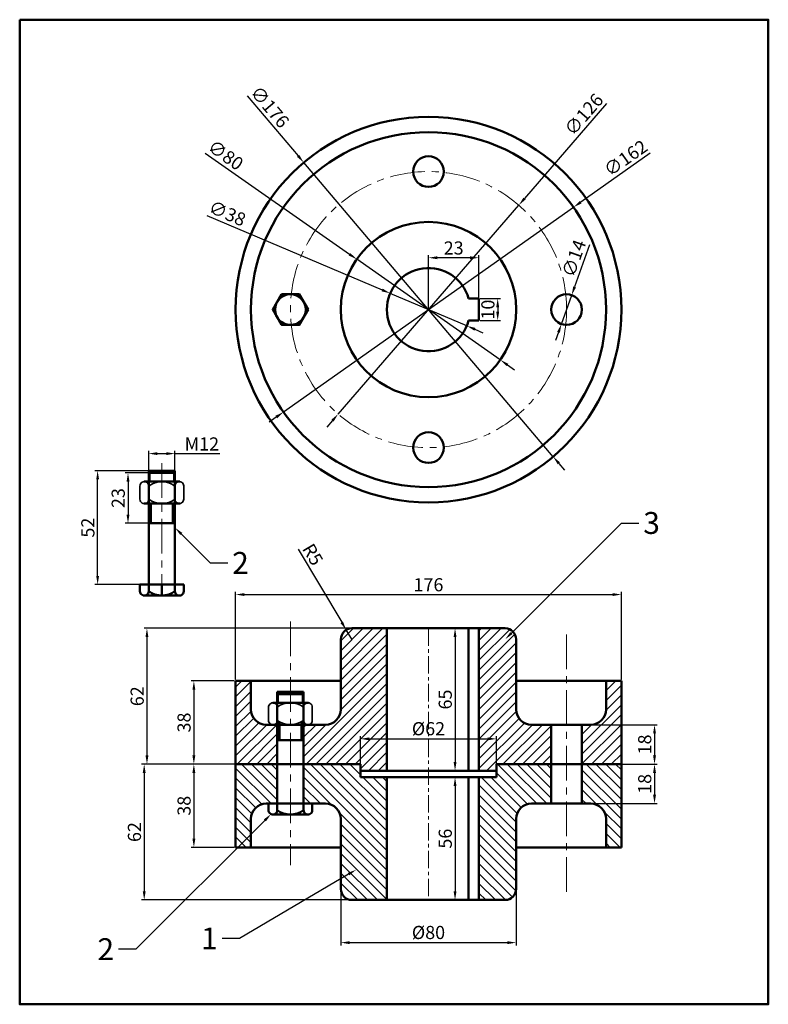
# Model space of a CAD drawing. Units: millimetres. Extents: x 50 to 392, y -77 to 372.
import ezdxf
from ezdxf import colors
from ezdxf.entities.mleader import LeaderData, LeaderLine
from ezdxf.math import Vec2, Vec3

# ---------------------------------------------------------------- set-up
doc = ezdxf.new("R2010")
doc.units = ezdxf.units.MM
doc.header["$LTSCALE"] = 0.5
doc.linetypes.add('CENTER', pattern=[50.8, 31.75, -6.35, 6.35, -6.35])
for name, color, linetype, lineweight in [('M-CNTR', 1, 'CENTER', 18), ('M-DIMS', 2, 'Continuous', 25), ('M-FAST', 4, 'Continuous', 35), ('M-HATC', 8, 'Continuous', 18), ('M-OUTL', 7, 'Continuous', 50), ('M-TEXT', 3, 'Continuous', 25), ('M-TTLB', 7, 'Continuous', 50)]:
    doc.layers.add(name, color=color, linetype=linetype, lineweight=lineweight)
doc.styles.get("Standard").update_dxf_attribs({"font": 'arial.ttf'})
doc.dimstyles.new('ISO-25', dxfattribs={"dimtxt": 6, "dimasz": 4, "dimexe": 1.25, "dimexo": 0.625, "dimtad": 1, "dimtxsty": 'Standard', "dimcen": 2.5, "dimadec": 0, "dimazin": 0, "dimtfac": 1, "dimtmove": 0, "dimatfit": 3, "dimfxl": 1, "dimarcsym": 0})

# ---------------------------------------------------------------- blocks, each defined once
blk = doc.blocks.new('*U1')
at = {"layer": 'M-CNTR', "color": 0, "transparency": 16777216}
blk.add_line((0, -62.78), (0, 57.14), dxfattribs=at)
blk = doc.blocks.new('*U2')
at = {"layer": 'M-CNTR', "color": 0, "transparency": 16777216}
blk.add_line((0, 29.5), (0, -29.5), dxfattribs=at)
blk = doc.blocks.new('*U3')
at = {"layer": 'M-CNTR', "color": 0, "transparency": 16777216}
blk.add_line((0, 57.63), (0, -53.66), dxfattribs=at)
blk = doc.blocks.new('*D4')
at = {"layer": 'Defpoints', "color": 0, "ltscale": 0.5, "transparency": 16777216}
for p in [(85.73, 166.64), (115.03, 166.64), (115.03, 114.64)]:
    blk.add_point(p, dxfattribs=at)
at = {"layer": 'M-DIMS', "color": 0, "lineweight": -2, "ltscale": 0.5, "transparency": 16777216}
for p, q in [((114.41, 166.64), (84.48, 166.64)), ((85.73, 118.64), (85.73, 162.64)), ((114.41, 114.64), (84.48, 114.64))]:
    blk.add_line(p, q, dxfattribs=at)
at = {"layer": 'M-DIMS', "color": 0, "ltscale": 0.5, "transparency": 16777216}
for points in [[(85.07, 162.64), (86.4, 162.64), (85.73, 166.64)], [(85.07, 118.64), (86.4, 118.64), (85.73, 114.64)]]:
    blk.add_solid(points, dxfattribs=at)
at = {"layer": 'M-DIMS', "color": 0, "ltscale": 0.5, "transparency": 16777216, "insert": (82.05, 140.64), "char_height": 6, "attachment_point": 5, "rotation": 90}
blk.add_mtext('52', dxfattribs=at)
blk = doc.blocks.new('*D5')
at = {"layer": 'Defpoints', "color": 0, "ltscale": 0.5, "transparency": 16777216}
for p in [(115.03, 165.64), (99.59, 142.64), (115.03, 142.64)]:
    blk.add_point(p, dxfattribs=at)
at = {"layer": 'M-DIMS', "color": 0, "lineweight": -2, "ltscale": 0.5, "transparency": 16777216}
for p, q in [((114.41, 165.64), (98.34, 165.64)), ((99.59, 161.64), (99.59, 146.64)), ((114.41, 142.64), (98.34, 142.64))]:
    blk.add_line(p, q, dxfattribs=at)
at = {"layer": 'M-DIMS', "color": 0, "ltscale": 0.5, "transparency": 16777216}
for points in [[(98.93, 161.64), (100.26, 161.64), (99.59, 165.64)], [(98.93, 146.64), (100.26, 146.64), (99.59, 142.64)]]:
    blk.add_solid(points, dxfattribs=at)
at = {"layer": 'M-DIMS', "color": 0, "ltscale": 0.5, "transparency": 16777216, "insert": (95.9, 154.14), "char_height": 6, "attachment_point": 5, "rotation": 90}
blk.add_mtext('23', dxfattribs=at)
blk = doc.blocks.new('*D6')
at = {"layer": 'Defpoints', "color": 0, "ltscale": 0.5, "transparency": 16777216}
for p in [(121.03, 174.43), (109.03, 161.64), (121.03, 161.64)]:
    blk.add_point(p, dxfattribs=at)
at = {"layer": 'M-DIMS', "color": 0, "lineweight": -2, "ltscale": 0.5, "transparency": 16777216}
for p, q in [((109.03, 162.26), (109.03, 175.68)), ((121.03, 162.26), (121.03, 175.68)), ((113.03, 174.43), (117.03, 174.43)), ((121.03, 174.43), (141.52, 174.43))]:
    blk.add_line(p, q, dxfattribs=at)
at = {"layer": 'M-DIMS', "color": 0, "ltscale": 0.5, "transparency": 16777216}
for points in [[(113.03, 175.1), (113.03, 173.76), (109.03, 174.43)], [(117.03, 175.1), (117.03, 173.76), (121.03, 174.43)]]:
    blk.add_solid(points, dxfattribs=at)
at = {"layer": 'M-DIMS', "color": 0, "ltscale": 0.5, "transparency": 16777216, "insert": (133.28, 178.07), "char_height": 6, "attachment_point": 5}
blk.add_mtext('M12', dxfattribs=at)
blk = doc.blocks.new('*D7')
at = {"layer": 'Defpoints', "color": 0, "ltscale": 0.5, "transparency": 16777216}
for p in [(236.69, 263.84), (236.69, 240.17), (259.69, 240.17)]:
    blk.add_point(p, dxfattribs=at)
at = {"layer": 'M-DIMS', "color": 0, "lineweight": -2, "ltscale": 0.5, "transparency": 16777216}
for p, q in [((236.69, 240.79), (236.69, 265.09)), ((255.69, 263.84), (240.69, 263.84)), ((259.69, 240.79), (259.69, 265.09))]:
    blk.add_line(p, q, dxfattribs=at)
at = {"layer": 'M-DIMS', "color": 0, "ltscale": 0.5, "transparency": 16777216}
for points in [[(240.69, 264.51), (240.69, 263.17), (236.69, 263.84)], [(255.69, 264.51), (255.69, 263.17), (259.69, 263.84)]]:
    blk.add_solid(points, dxfattribs=at)
at = {"layer": 'M-DIMS', "color": 0, "ltscale": 0.5, "transparency": 16777216, "insert": (248.19, 267.53), "char_height": 6, "attachment_point": 5}
blk.add_mtext('23', dxfattribs=at)
blk = doc.blocks.new('*D8')
at = {"layer": 'Defpoints', "color": 0, "ltscale": 0.5, "transparency": 16777216}
for p in [(302.86, 286.88), (170.52, 193.45)]:
    blk.add_point(p, dxfattribs=at)
at = {"layer": 'M-DIMS', "color": 0, "lineweight": -2, "ltscale": 0.5, "transparency": 16777216}
for p, q in [((337.9, 311.62), (306.13, 289.19)), ((170.52, 193.45), (302.86, 286.88)), ((167.25, 191.14), (163.99, 188.84))]:
    blk.add_line(p, q, dxfattribs=at)
at = {"layer": 'M-DIMS', "color": 0, "ltscale": 0.5, "transparency": 16777216}
for points in [[(305.75, 289.73), (306.51, 288.65), (302.86, 286.88)], [(166.87, 191.69), (167.64, 190.6), (170.52, 193.45)]]:
    blk.add_solid(points, dxfattribs=at)
at = {"layer": 'M-DIMS', "color": 0, "ltscale": 0.5, "transparency": 16777216, "insert": (327.11, 308.72), "char_height": 6, "attachment_point": 5, "rotation": 35.2225}
blk.add_mtext('∅162', dxfattribs=at)
blk = doc.blocks.new('*D9')
at = {"layer": 'Defpoints', "color": 0, "ltscale": 0.5, "transparency": 16777216}
for p in [(179.79, 307.29), (293.59, 173.04)]:
    blk.add_point(p, dxfattribs=at)
at = {"layer": 'M-DIMS', "color": 0, "lineweight": -2, "ltscale": 0.5, "transparency": 16777216}
for p, q in [((153.99, 337.73), (177.2, 310.35)), ((293.59, 173.04), (179.79, 307.29)), ((296.18, 169.99), (298.77, 166.94))]:
    blk.add_line(p, q, dxfattribs=at)
at = {"layer": 'M-DIMS', "color": 0, "ltscale": 0.5, "transparency": 16777216}
for points in [[(177.71, 310.78), (176.7, 309.91), (179.79, 307.29)], [(296.69, 170.42), (295.67, 169.56), (293.59, 173.04)]]:
    blk.add_solid(points, dxfattribs=at)
at = {"layer": 'M-DIMS', "color": 0, "ltscale": 0.5, "transparency": 16777216, "insert": (163.73, 332.2), "char_height": 6, "attachment_point": 5, "rotation": 310.2866}
blk.add_mtext('∅176', dxfattribs=at)
blk = doc.blocks.new('*D10')
at = {"layer": 'Defpoints', "color": 0, "ltscale": 0.5, "transparency": 16777216}
for p in [(277.89, 287.83), (195.49, 192.51)]:
    blk.add_point(p, dxfattribs=at)
at = {"layer": 'M-DIMS', "color": 0, "lineweight": -2, "ltscale": 0.5, "transparency": 16777216}
for p, q in [((317.96, 334.17), (280.51, 290.85)), ((195.49, 192.51), (277.89, 287.83)), ((192.87, 189.48), (190.26, 186.46))]:
    blk.add_line(p, q, dxfattribs=at)
at = {"layer": 'M-DIMS', "color": 0, "ltscale": 0.5, "transparency": 16777216}
for points in [[(280.01, 291.29), (281.01, 290.42), (277.89, 287.83)], [(192.37, 189.92), (193.38, 189.05), (195.49, 192.51)]]:
    blk.add_solid(points, dxfattribs=at)
at = {"layer": 'M-DIMS', "color": 0, "ltscale": 0.5, "transparency": 16777216, "insert": (308.17, 328.74), "char_height": 6, "attachment_point": 5, "rotation": 49.1562}
blk.add_mtext('∅126', dxfattribs=at)
blk = doc.blocks.new('*D11')
at = {"layer": 'Defpoints', "color": 0, "ltscale": 0.5, "transparency": 16777216}
for p in [(203.94, 263.13), (269.45, 217.21)]:
    blk.add_point(p, dxfattribs=at)
at = {"layer": 'M-DIMS', "color": 0, "lineweight": -2, "ltscale": 0.5, "transparency": 16777216}
for p, q in [((134.77, 311.61), (200.66, 265.42)), ((269.45, 217.21), (203.94, 263.13)), ((272.72, 214.91), (276, 212.61))]:
    blk.add_line(p, q, dxfattribs=at)
at = {"layer": 'M-DIMS', "color": 0, "ltscale": 0.5, "transparency": 16777216}
for points in [[(201.05, 265.97), (200.28, 264.88), (203.94, 263.13)], [(273.1, 215.46), (272.34, 214.36), (269.45, 217.21)]]:
    blk.add_solid(points, dxfattribs=at)
at = {"layer": 'M-DIMS', "color": 0, "ltscale": 0.5, "transparency": 16777216, "insert": (143.68, 310.07), "char_height": 6, "attachment_point": 5, "rotation": 324.9705}
blk.add_mtext('∅80', dxfattribs=at)
blk = doc.blocks.new('*D12')
at = {"layer": 'Defpoints', "color": 0, "ltscale": 0.5, "transparency": 16777216}
for p in [(219.2, 247.58), (254.18, 232.75)]:
    blk.add_point(p, dxfattribs=at)
at = {"layer": 'M-DIMS', "color": 0, "lineweight": -2, "ltscale": 0.5, "transparency": 16777216}
for p, q in [((135.55, 283.05), (215.52, 249.14)), ((254.18, 232.75), (219.2, 247.58)), ((257.87, 231.19), (261.55, 229.63))]:
    blk.add_line(p, q, dxfattribs=at)
at = {"layer": 'M-DIMS', "color": 0, "ltscale": 0.5, "transparency": 16777216}
for points in [[(215.78, 249.76), (215.26, 248.53), (219.2, 247.58)], [(258.13, 231.8), (257.61, 230.57), (254.18, 232.75)]]:
    blk.add_solid(points, dxfattribs=at)
at = {"layer": 'M-DIMS', "color": 0, "ltscale": 0.5, "transparency": 16777216, "insert": (144.6, 283.4), "char_height": 6, "attachment_point": 5, "rotation": 337.0239}
blk.add_mtext('∅38', dxfattribs=at)
blk = doc.blocks.new('*D13')
at = {"layer": 'Defpoints', "color": 0, "ltscale": 0.5, "transparency": 16777216}
for p in [(259.69, 245.17), (259.69, 235.17), (268.27, 235.17)]:
    blk.add_point(p, dxfattribs=at)
at = {"layer": 'M-DIMS', "color": 0, "lineweight": -2, "ltscale": 0.5, "transparency": 16777216}
for p, q in [((260.32, 245.17), (269.52, 245.17)), ((268.27, 241.17), (268.27, 239.17)), ((260.32, 235.17), (269.52, 235.17))]:
    blk.add_line(p, q, dxfattribs=at)
at = {"layer": 'M-DIMS', "color": 0, "ltscale": 0.5, "transparency": 16777216}
for points in [[(267.6, 241.17), (268.94, 241.17), (268.27, 245.17)], [(267.6, 239.17), (268.94, 239.17), (268.27, 235.17)]]:
    blk.add_solid(points, dxfattribs=at)
at = {"layer": 'M-DIMS', "color": 0, "ltscale": 0.5, "transparency": 16777216, "insert": (264.58, 240.17), "char_height": 6, "attachment_point": 5, "rotation": 90}
blk.add_mtext('10', dxfattribs=at)
blk = doc.blocks.new('*D14')
at = {"layer": 'Defpoints', "color": 0, "ltscale": 0.5, "transparency": 16777216}
for p in [(302.03, 246.76), (297.35, 233.57)]:
    blk.add_point(p, dxfattribs=at)
at = {"layer": 'M-DIMS', "color": 0, "lineweight": -2, "ltscale": 0.5, "transparency": 16777216}
for p, q in [((310.16, 269.71), (303.37, 250.53)), ((297.35, 233.57), (302.03, 246.76)), ((296.02, 229.8), (294.68, 226.03))]:
    blk.add_line(p, q, dxfattribs=at)
at = {"layer": 'M-DIMS', "color": 0, "ltscale": 0.5, "transparency": 16777216}
for points in [[(302.74, 250.76), (303.99, 250.31), (302.03, 246.76)], [(295.39, 230.02), (296.65, 229.58), (297.35, 233.57)]]:
    blk.add_solid(points, dxfattribs=at)
at = {"layer": 'M-DIMS', "color": 0, "ltscale": 0.5, "transparency": 16777216, "insert": (303.8, 263.3), "char_height": 6, "attachment_point": 5, "rotation": 70.4869}
blk.add_mtext('∅14', dxfattribs=at)
blk = doc.blocks.new('*D15')
at = {"layer": 'Defpoints', "color": 0, "ltscale": 0.5, "transparency": 16777216}
for p in [(324.69, 110.11), (148.69, 70.69), (324.69, 70.69)]:
    blk.add_point(p, dxfattribs=at)
at = {"layer": 'M-DIMS', "color": 0, "lineweight": -2, "ltscale": 0.5, "transparency": 16777216}
for p, q in [((148.69, 71.31), (148.69, 111.36)), ((152.69, 110.11), (320.69, 110.11)), ((324.69, 71.31), (324.69, 111.36))]:
    blk.add_line(p, q, dxfattribs=at)
at = {"layer": 'M-DIMS', "color": 0, "ltscale": 0.5, "transparency": 16777216}
for points in [[(152.69, 110.77), (152.69, 109.44), (148.69, 110.11)], [(320.69, 110.77), (320.69, 109.44), (324.69, 110.11)]]:
    blk.add_solid(points, dxfattribs=at)
at = {"layer": 'M-DIMS', "color": 0, "ltscale": 0.5, "transparency": 16777216, "insert": (236.69, 113.8), "char_height": 6, "attachment_point": 5}
blk.add_mtext('176', dxfattribs=at)
blk = doc.blocks.new('*D16')
at = {"layer": 'Defpoints', "color": 0, "ltscale": 0.5, "transparency": 16777216}
for p in [(148.69, 70.69), (129.65, 32.69), (148.69, 32.69)]:
    blk.add_point(p, dxfattribs=at)
at = {"layer": 'M-DIMS', "color": 0, "lineweight": -2, "ltscale": 0.5, "transparency": 16777216}
for p, q in [((148.07, 70.69), (128.4, 70.69)), ((129.65, 66.69), (129.65, 36.69)), ((148.07, 32.69), (128.4, 32.69))]:
    blk.add_line(p, q, dxfattribs=at)
at = {"layer": 'M-DIMS', "color": 0, "ltscale": 0.5, "transparency": 16777216}
for points in [[(128.98, 66.69), (130.31, 66.69), (129.65, 70.69)], [(128.98, 36.69), (130.31, 36.69), (129.65, 32.69)]]:
    blk.add_solid(points, dxfattribs=at)
at = {"layer": 'M-DIMS', "color": 0, "ltscale": 0.5, "transparency": 16777216, "insert": (125.95, 51.69), "char_height": 6, "attachment_point": 5, "rotation": 90}
blk.add_mtext('38', dxfattribs=at)
blk = doc.blocks.new('*D17')
at = {"layer": 'Defpoints', "color": 0, "ltscale": 0.5, "transparency": 16777216}
for p in [(138.23, 32.69), (129.65, -5.31), (148.69, -5.31)]:
    blk.add_point(p, dxfattribs=at)
at = {"layer": 'M-DIMS', "color": 0, "lineweight": -2, "ltscale": 0.5, "transparency": 16777216}
for p, q in [((137.61, 32.69), (128.4, 32.69)), ((129.65, 28.69), (129.65, -1.31)), ((148.07, -5.31), (128.4, -5.31))]:
    blk.add_line(p, q, dxfattribs=at)
at = {"layer": 'M-DIMS', "color": 0, "ltscale": 0.5, "transparency": 16777216}
for points in [[(128.98, 28.69), (130.31, 28.69), (129.65, 32.69)], [(128.98, -1.31), (130.31, -1.31), (129.65, -5.31)]]:
    blk.add_solid(points, dxfattribs=at)
at = {"layer": 'M-DIMS', "color": 0, "ltscale": 0.5, "transparency": 16777216, "insert": (125.95, 13.69), "char_height": 6, "attachment_point": 5, "rotation": 90}
blk.add_mtext('38', dxfattribs=at)
blk = doc.blocks.new('*D18')
at = {"layer": 'Defpoints', "color": 0, "ltscale": 0.5, "transparency": 16777216}
for p in [(306.69, 50.69), (306.69, 32.69), (339.83, 32.69)]:
    blk.add_point(p, dxfattribs=at)
at = {"layer": 'M-DIMS', "color": 0, "lineweight": -2, "ltscale": 0.5, "transparency": 16777216}
for p, q in [((307.32, 50.69), (341.08, 50.69)), ((339.83, 46.69), (339.83, 36.69)), ((307.32, 32.69), (341.08, 32.69))]:
    blk.add_line(p, q, dxfattribs=at)
at = {"layer": 'M-DIMS', "color": 0, "ltscale": 0.5, "transparency": 16777216}
for points in [[(339.16, 46.69), (340.49, 46.69), (339.83, 50.69)], [(339.16, 36.69), (340.49, 36.69), (339.83, 32.69)]]:
    blk.add_solid(points, dxfattribs=at)
at = {"layer": 'M-DIMS', "color": 0, "ltscale": 0.5, "transparency": 16777216, "insert": (336.14, 41.69), "char_height": 6, "attachment_point": 5, "rotation": 90}
blk.add_mtext('18', dxfattribs=at)
blk = doc.blocks.new('*D19')
at = {"layer": 'Defpoints', "color": 0, "ltscale": 0.5, "transparency": 16777216}
for p in [(306.69, 32.69), (306.69, 14.69), (339.83, 14.69)]:
    blk.add_point(p, dxfattribs=at)
at = {"layer": 'M-DIMS', "color": 0, "lineweight": -2, "ltscale": 0.5, "transparency": 16777216}
for p, q in [((307.32, 32.69), (341.08, 32.69)), ((339.83, 28.69), (339.83, 18.69)), ((307.32, 14.69), (341.08, 14.69))]:
    blk.add_line(p, q, dxfattribs=at)
at = {"layer": 'M-DIMS', "color": 0, "ltscale": 0.5, "transparency": 16777216}
for points in [[(339.16, 28.69), (340.49, 28.69), (339.83, 32.69)], [(339.16, 18.69), (340.49, 18.69), (339.83, 14.69)]]:
    blk.add_solid(points, dxfattribs=at)
at = {"layer": 'M-DIMS', "color": 0, "ltscale": 0.5, "transparency": 16777216, "insert": (336.14, 23.69), "char_height": 6, "attachment_point": 5, "rotation": 90}
blk.add_mtext('18', dxfattribs=at)
blk = doc.blocks.new('*D20')
at = {"layer": 'Defpoints', "color": 0, "ltscale": 0.5, "transparency": 16777216}
for p in [(245.13, 94.69), (245.13, 29.69), (248.81, 29.69)]:
    blk.add_point(p, dxfattribs=at)
at = {"layer": 'M-DIMS', "color": 0, "lineweight": -2, "ltscale": 0.5, "transparency": 16777216}
for p, q in [((245.75, 94.69), (250.06, 94.69)), ((248.81, 90.69), (248.81, 33.69)), ((245.75, 29.69), (250.06, 29.69))]:
    blk.add_line(p, q, dxfattribs=at)
at = {"layer": 'M-DIMS', "color": 0, "ltscale": 0.5, "transparency": 16777216}
for points in [[(248.14, 90.69), (249.48, 90.69), (248.81, 94.69)], [(248.14, 33.69), (249.48, 33.69), (248.81, 29.69)]]:
    blk.add_solid(points, dxfattribs=at)
at = {"layer": 'M-DIMS', "color": 0, "ltscale": 0.5, "transparency": 16777216, "insert": (245.12, 62.19), "char_height": 6, "attachment_point": 5, "rotation": 90}
blk.add_mtext('65', dxfattribs=at)
blk = doc.blocks.new('*D21')
at = {"layer": 'Defpoints', "color": 0, "ltscale": 0.5, "transparency": 16777216}
for p in [(248.81, 26.69), (248.81, -29.31), (248.81, -29.31)]:
    blk.add_point(p, dxfattribs=at)
at = {"layer": 'M-DIMS', "color": 0, "lineweight": -2, "ltscale": 0.5, "transparency": 16777216}
for p, q in [((248.81, 22.69), (248.81, -25.31)), ((249.43, 26.69), (250.06, 26.69)), ((249.43, -29.31), (250.06, -29.31))]:
    blk.add_line(p, q, dxfattribs=at)
at = {"layer": 'M-DIMS', "color": 0, "ltscale": 0.5, "transparency": 16777216}
for points in [[(248.14, 22.69), (249.48, 22.69), (248.81, 26.69)], [(248.14, -25.31), (249.48, -25.31), (248.81, -29.31)]]:
    blk.add_solid(points, dxfattribs=at)
at = {"layer": 'M-DIMS', "color": 0, "ltscale": 0.5, "transparency": 16777216, "insert": (245.12, -1.31), "char_height": 6, "attachment_point": 5, "rotation": 90}
blk.add_mtext('56', dxfattribs=at)
blk = doc.blocks.new('*D22')
at = {"layer": 'Defpoints', "color": 0, "ltscale": 0.5, "transparency": 16777216}
for p in [(267.69, 44.23), (205.69, 28.19), (267.69, 28.19)]:
    blk.add_point(p, dxfattribs=at)
at = {"layer": 'M-DIMS', "color": 0, "lineweight": -2, "ltscale": 0.5, "transparency": 16777216}
for p, q in [((205.69, 28.81), (205.69, 45.48)), ((267.69, 28.81), (267.69, 45.48)), ((209.69, 44.23), (263.69, 44.23))]:
    blk.add_line(p, q, dxfattribs=at)
at = {"layer": 'M-DIMS', "color": 0, "ltscale": 0.5, "transparency": 16777216}
for points in [[(209.69, 44.9), (209.69, 43.57), (205.69, 44.23)], [(263.69, 44.9), (263.69, 43.57), (267.69, 44.23)]]:
    blk.add_solid(points, dxfattribs=at)
at = {"layer": 'M-DIMS', "color": 0, "ltscale": 0.5, "transparency": 16777216, "insert": (236.69, 48.09), "char_height": 6, "attachment_point": 5}
blk.add_mtext('%%C62', dxfattribs=at)
blk = doc.blocks.new('*D23')
at = {"layer": 'Defpoints', "color": 0, "ltscale": 0.5, "transparency": 16777216}
for p in [(217.69, 94.69), (108.24, 32.69), (198.69, 32.69)]:
    blk.add_point(p, dxfattribs=at)
at = {"layer": 'M-DIMS', "color": 0, "lineweight": -2, "ltscale": 0.5, "transparency": 16777216}
for p, q in [((217.07, 94.69), (106.99, 94.69)), ((108.24, 90.69), (108.24, 36.69)), ((198.06, 32.69), (106.99, 32.69))]:
    blk.add_line(p, q, dxfattribs=at)
at = {"layer": 'M-DIMS', "color": 0, "ltscale": 0.5, "transparency": 16777216}
for points in [[(107.57, 90.69), (108.9, 90.69), (108.24, 94.69)], [(107.57, 36.69), (108.9, 36.69), (108.24, 32.69)]]:
    blk.add_solid(points, dxfattribs=at)
at = {"layer": 'M-DIMS', "color": 0, "ltscale": 0.5, "transparency": 16777216, "insert": (104.55, 63.69), "char_height": 6, "attachment_point": 5, "rotation": 90}
blk.add_mtext('62', dxfattribs=at)
blk = doc.blocks.new('*D24')
at = {"layer": 'Defpoints', "color": 0, "ltscale": 0.5, "transparency": 16777216}
for p in [(122.27, 32.69), (106.99, -29.31), (226.18, -29.31)]:
    blk.add_point(p, dxfattribs=at)
at = {"layer": 'M-DIMS', "color": 0, "lineweight": -2, "ltscale": 0.5, "transparency": 16777216}
for p, q in [((121.64, 32.69), (105.74, 32.69)), ((106.99, 28.69), (106.99, -25.31)), ((225.55, -29.31), (105.74, -29.31))]:
    blk.add_line(p, q, dxfattribs=at)
at = {"layer": 'M-DIMS', "color": 0, "ltscale": 0.5, "transparency": 16777216}
for points in [[(106.32, 28.69), (107.65, 28.69), (106.99, 32.69)], [(106.32, -25.31), (107.65, -25.31), (106.99, -29.31)]]:
    blk.add_solid(points, dxfattribs=at)
at = {"layer": 'M-DIMS', "color": 0, "ltscale": 0.5, "transparency": 16777216, "insert": (103.3, 1.69), "char_height": 6, "attachment_point": 5, "rotation": 90}
blk.add_mtext('62', dxfattribs=at)
blk = doc.blocks.new('*D25')
at = {"layer": 'Defpoints', "color": 0, "ltscale": 0.5, "transparency": 16777216}
for p in [(196.69, -15.83), (276.69, -15.83), (276.69, -48.78)]:
    blk.add_point(p, dxfattribs=at)
at = {"layer": 'M-DIMS', "color": 0, "lineweight": -2, "ltscale": 0.5, "transparency": 16777216}
for p, q in [((196.69, -16.46), (196.69, -50.03)), ((276.69, -16.46), (276.69, -50.03)), ((200.69, -48.78), (272.69, -48.78))]:
    blk.add_line(p, q, dxfattribs=at)
at = {"layer": 'M-DIMS', "color": 0, "ltscale": 0.5, "transparency": 16777216}
for points in [[(200.69, -48.11), (200.69, -49.45), (196.69, -48.78)], [(272.69, -48.11), (272.69, -49.45), (276.69, -48.78)]]:
    blk.add_solid(points, dxfattribs=at)
at = {"layer": 'M-DIMS', "color": 0, "ltscale": 0.5, "transparency": 16777216, "insert": (236.69, -44.92), "char_height": 6, "attachment_point": 5}
blk.add_mtext('%%C80', dxfattribs=at)
blk = doc.blocks.new('*D26')
at = {"layer": 'Defpoints', "color": 0, "ltscale": 0.5, "transparency": 16777216}
for p in [(199.14, 93.99), (201.69, 89.69)]:
    blk.add_point(p, dxfattribs=at)
at = {"layer": 'M-DIMS', "color": 0, "lineweight": -2, "ltscale": 0.5, "transparency": 16777216}
for p, q in [((177.28, 130.82), (197.1, 97.43)), ((201.69, 89.69), (199.14, 93.99))]:
    blk.add_line(p, q, dxfattribs=at)
at = {"layer": 'M-DIMS', "color": 0, "ltscale": 0.5, "transparency": 16777216}
blk.add_solid([(197.67, 97.77), (196.53, 97.09), (199.14, 93.99)], dxfattribs=at)
at = {"layer": 'M-DIMS', "color": 0, "ltscale": 0.5, "transparency": 16777216, "insert": (183.24, 127.98), "char_height": 6, "attachment_point": 5, "rotation": 300.6854}
blk.add_mtext('R5', dxfattribs=at)
blk = doc.blocks.new('NUT-HEX')
at = {"ltscale": 0.5}
for p, q in [((0, 8.01), (0, 2.01)), ((4, 8.01), (4, 2.01)), ((16, 8.03), (16, 1.99)), ((20, 8.03), (20, 1.99))]:
    blk.add_line(p, q, dxfattribs=at)
for centre, radius, start, end in [((2, 8.01), 2, 359.9944, 180.0056), ((10, 0.01), 10, 53.1316, 126.8647), ((18, 8.02), 2, 359.7093, 180.2906), ((2, 2.01), 2, 179.9944, 0.0056), ((10, 10.01), 10, 233.1353, 306.8684), ((18, 2), 2, 179.7094, 0.2907)]:
    blk.add_arc(centre, radius, start, end, dxfattribs=at)

msp = doc.modelspace()

# ---------------------------------------------------------------- hatches: boundary and pattern name
at = {"layer": 'M-HATC', "ltscale": 0.5}
h = msp.add_hatch(dxfattribs=at)
h.set_pattern_fill('ANSI31', color=256)
h.paths.add_polyline_path([(292.692, 50.687), (283.692, 50.687, -0.4142136), (276.692, 57.687), (276.692, 89.687, 0.4142136), (271.692, 94.687), (259.692, 94.687), (259.692, 29.687), (267.692, 29.687), (267.692, 32.687), (292.692, 32.687)])
h.paths.add_polyline_path([(324.692, 70.687), (317.692, 70.687), (317.692, 57.687, -0.4142136), (310.692, 50.687), (306.692, 50.687), (306.692, 32.687), (324.692, 32.687)])
h.paths.add_polyline_path([(217.692, 94.687), (201.692, 94.687, 0.4142136), (196.692, 89.687), (196.692, 57.687, -0.4142136), (189.692, 50.687), (181.894, 50.687, -0.0504915), (181.491, 50.687), (179.692, 50.687), (179.692, 32.687), (205.692, 32.687), (205.692, 29.687), (217.692, 29.687)])
h.paths.add_polyline_path([(167.692, 50.687), (162.692, 50.687, -0.4142136), (155.692, 57.687), (155.692, 70.687), (148.692, 70.687), (148.692, 32.687), (167.692, 32.687)])
h = msp.add_hatch(dxfattribs=at)
h.set_pattern_fill('ANSI31', color=256, angle=90)
h.paths.add_polyline_path([(217.692, 26.687), (205.692, 26.687), (205.692, 29.687), (205.692, 32.687), (179.692, 32.687), (179.692, 14.687), (189.692, 14.687, -0.4142136), (196.692, 7.687), (196.692, -24.313, 0.4142136), (201.692, -29.313), (217.692, -29.313)])
h.paths.add_polyline_path([(167.692, 32.687), (148.692, 32.687), (148.692, -5.313), (155.692, -5.313), (155.692, 7.687, -0.4142136), (162.692, 14.687), (167.692, 14.687)])
h.paths.add_polyline_path([(292.692, 32.687), (267.692, 32.687), (267.692, 29.687), (267.692, 26.687), (259.692, 26.687), (259.692, -29.313), (271.692, -29.313, 0.4142136), (276.692, -24.313), (276.692, 7.687, -0.4142136), (283.692, 14.687), (292.692, 14.687)])
h.paths.add_polyline_path([(324.692, 32.687), (306.692, 32.687), (306.692, 14.687), (310.692, 14.687, -0.4142136), (317.692, 7.687), (317.692, -5.313), (324.692, -5.313)])

# ---------------------------------------------------------------- linework, layer by layer
at = {"layer": 'M-CNTR', "ltscale": 0.5}
msp.add_line((236.692, 94.687), (236.692, -29.313), dxfattribs=at)
at = {"layer": 'M-CNTR'}
msp.add_circle((236.692, 240.166), 63, dxfattribs=at)
at = {"layer": 'M-OUTL'}
for p, q in [((259.692, 245.166), (255.022, 245.166)), ((259.692, 240.166), (259.692, 245.166)), ((259.692, 240.166), (259.692, 235.166)), ((259.692, 235.166), (255.022, 235.166)), ((201.692, 94.687), (271.692, 94.687)), ((196.692, 57.687), (196.692, 89.687)), ((276.692, 57.687), (276.692, 89.687)), ((148.692, -5.313), (148.692, 70.687)), ((148.692, 70.687), (196.692, 70.687)), ((155.692, 57.687), (155.692, 70.687)), ((276.692, 70.687), (324.692, 70.687)), ((317.692, 70.687), (317.692, 57.687)), ((324.692, 70.687), (324.692, -5.313)), ((148.692, 32.687), (205.692, 32.687)), ((267.692, 32.687), (324.692, 32.687)), ((155.692, -5.313), (155.692, 7.687)), ((196.692, -24.313), (196.692, 7.687)), ((276.692, -24.313), (276.692, 7.687)), ((317.692, 7.687), (317.692, -5.313)), ((148.692, -5.313), (196.692, -5.313)), ((276.692, -5.313), (324.692, -5.313)), ((271.692, -29.313), (201.692, -29.313))]:
    msp.add_line(p, q, dxfattribs=at)
at = {"layer": 'M-OUTL', "ltscale": 0.5}
for p, q in [((109.03, 166.636), (121.03, 166.636)), ((109.03, 166.636), (109.03, 114.636)), ((109.34, 161.636), (109.34, 166.636)), ((120.721, 166.636), (120.721, 161.636)), ((121.03, 166.636), (121.03, 114.636)), ((109.03, 165.636), (121.03, 165.636)), ((123.232, 161.636), (107.002, 161.636)), ((107.002, 151.636), (123.232, 151.636)), ((110.03, 151.636), (110.03, 142.636)), ((120.03, 151.637), (120.03, 142.637)), ((109.03, 142.636), (121.03, 142.636)), ((105.03, 114.636), (105.03, 111.636)), ((105.03, 114.636), (125.03, 114.636)), ((109.03, 114.636), (109.03, 111.636)), ((115.03, 114.636), (115.03, 109.636)), ((121.03, 114.636), (121.03, 111.616)), ((125.03, 114.636), (125.03, 111.616)), ((107.002, 109.636), (123.232, 109.636)), ((217.692, 94.687), (217.692, 29.687)), ((255.022, 94.687), (255.022, 29.687)), ((259.692, 94.687), (259.692, 29.687)), ((167.692, 65.687), (179.692, 65.687)), ((167.692, 65.687), (167.692, 14.687)), ((168.002, 60.687), (168.002, 65.687)), ((168.002, 64.687), (179.382, 64.687)), ((179.382, 65.687), (179.382, 60.687)), ((179.692, 65.687), (179.692, 14.687)), ((181.894, 60.687), (165.664, 60.687)), ((162.692, 50.687), (189.692, 50.687)), ((168.692, 52.026), (168.692, 43.687)), ((178.692, 52.026), (178.692, 43.687)), ((310.692, 50.687), (283.692, 50.687)), ((292.692, 50.687), (292.692, 14.687)), ((306.692, 32.687), (306.692, 50.687)), ((167.692, 43.687), (179.692, 43.687)), ((205.692, 29.687), (205.692, 32.687)), ((267.692, 29.687), (267.692, 32.687)), ((306.692, 14.687), (306.692, 32.687)), ((205.692, 29.687), (267.692, 29.687)), ((205.692, 26.687), (205.692, 29.687)), ((267.692, 29.687), (267.692, 26.687)), ((267.692, 26.687), (205.692, 26.687)), ((217.692, 26.687), (217.692, -29.313)), ((255.022, 26.687), (255.022, -29.313)), ((259.692, 26.687), (259.692, -29.313)), ((162.692, 14.687), (189.692, 14.687)), ((163.692, 14.687), (163.692, 11.686)), ((167.692, 14.687), (167.692, 11.686)), ((179.692, 14.687), (179.692, 11.666)), ((183.692, 14.687), (183.692, 11.666)), ((283.692, 14.687), (310.692, 14.687)), ((165.664, 9.687), (181.894, 9.687))]:
    msp.add_line(p, q, dxfattribs=at)
msp.add_lwpolyline([(169.651, 247.166), (165.609, 240.166), (169.651, 233.166), (177.734, 233.166), (181.775, 240.166), (177.734, 247.166)], close=True, dxfattribs=at)
at = {"layer": 'M-OUTL'}
for centre, radius in [((236.692, 240.166), 88), ((236.692, 240.166), 81), ((236.692, 303.166), 7), ((236.692, 240.166), 40), ((299.692, 240.166), 7), ((236.692, 177.166), 7)]:
    msp.add_circle(centre, radius, dxfattribs=at)
at = {"layer": 'M-OUTL', "ltscale": 0.5}
msp.add_circle((173.692, 240.166), 7, dxfattribs=at)
at = {"layer": 'M-OUTL'}
for centre, radius, start, end in [((236.692, 240.166), 19, 15.25752, 344.74248), ((201.692, 89.687), 5, 90, 180), ((271.692, 89.687), 5, 0, 90), ((189.692, 57.687), 7, 270, 360), ((162.692, 7.687), 7, 90, 180), ((189.692, 7.687), 7, 360, 90), ((283.692, 7.687), 7, 90, 180), ((310.692, 7.687), 7, 0, 90), ((201.692, -24.313), 5, 180, 270), ((271.692, -24.313), 5, 270, 0)]:
    msp.add_arc(centre, radius, start, end, dxfattribs=at)
at = {"layer": 'M-OUTL', "ltscale": 0.5}
for centre, radius, start, end in [((115.03, 149.947), 16.69, 70.0654, 109.9346), ((107.03, 111.636), 2, 179.99439, 0.00561), ((115.03, 119.637), 10.001, 233.13534, 306.8684), ((123.03, 111.626), 2, 179.70936, 0.29065), ((173.692, 48.997), 16.69, 70.0654, 109.9346), ((162.692, 57.687), 7, 180, 270), ((283.692, 57.687), 7, 180, 270), ((310.692, 57.687), 7, 270, 0), ((165.692, 11.686), 2, 179.99439, 0.00561), ((173.692, 19.687), 10.001, 233.13534, 306.8684), ((181.692, 11.677), 2, 179.70936, 0.29065)]:
    msp.add_arc(centre, radius, start, end, dxfattribs=at)
at = {"layer": 'M-TTLB', "ltscale": 0.5}
msp.add_lwpolyline([(50.174, 372.497), (391.739, 372.497), (391.739, -76.928), (50.174, -76.928)], close=True, dxfattribs=at)

# ---------------------------------------------------------------- block references
at = {"layer": 'M-CNTR'}
for name, p in [('*U2', (115.03, 140.636)), ('*U3', (173.692, 40.187)), ('*U1', (299.692, 37.187))]:
    msp.add_blockref(name, p, dxfattribs=at)
at = {"layer": 'M-FAST', "rotation": 180.104480186598}
msp.add_blockref('NUT-HEX', (125.021, 161.664), dxfattribs=at)
at = {"layer": 'M-FAST'}
msp.add_blockref('NUT-HEX', (163.692, 50.677), dxfattribs=at)

# ---------------------------------------------------------------- dimensions: what is measured, and where the dimension line sits
at = {"layer": 'M-DIMS', "ltscale": 0.5}
for p1, p2, picture, middle in [((293.594, 173.038), (179.79, 307.294), '*D9', (160.793, 329.706)), ((195.49, 192.507), (277.894, 287.826), '*D10', (311.087, 326.22)), ((269.446, 217.206), (203.938, 263.126), '*D11', (141.47, 306.915)), ((170.522, 193.449), (302.863, 286.883), '*D8', (329.336, 305.574)), ((254.185, 232.75), (219.199, 247.583), '*D12', (143.096, 279.849))]:
    dim = msp.add_diameter_dim_2p(p1=p1, p2=p2, dimstyle='ISO-25', override={"dimclrd": 0, "dimclre": 0, "dimclrt": 0}, dxfattribs=at)
    dim.commit()
    dim.dimension.update_dxf_attribs({"geometry": picture, "text_midpoint": middle, "dimtype": 163})
for base, p1, p2, picture, middle in [((236.692, 263.841), (259.692, 240.166), (236.692, 240.166), '*D7', (248.192, 267.531)), ((324.692, 110.108), (148.692, 70.687), (324.692, 70.687), '*D15', (236.692, 113.796))]:
    dim = msp.add_linear_dim(base=base, p1=p1, p2=p2, dimstyle='ISO-25', override={"dimclrd": 0, "dimclre": 0, "dimclrt": 0}, dxfattribs=at)
    dim.commit()
    dim.dimension.update_dxf_attribs({"geometry": picture, "text_midpoint": middle})
dim = msp.add_diameter_dim_2p(p1=(297.354, 233.568), p2=(302.03, 246.764), dimstyle='ISO-25', override={"dimclrd": 0, "dimclre": 0, "dimclrt": 0}, dxfattribs=at)
dim.commit()
dim.dimension.update_dxf_attribs({"geometry": '*D14', "text_midpoint": (303.798, 263.298)})
for base, p1, p2, picture, middle in [((268.271, 235.166), (259.692, 245.166), (259.692, 235.166), '*D13', (264.583, 240.166)), ((99.595, 142.636), (115.03, 165.636), (115.03, 142.636), '*D5', (95.904, 154.136)), ((248.81, 29.687), (245.127, 94.687), (245.127, 29.687), '*D20', (245.121, 62.187)), ((129.645, 32.687), (148.692, 70.687), (148.692, 32.687), '*D16', (125.955, 51.687)), ((339.826, 32.687), (306.692, 50.687), (306.692, 32.687), '*D18', (336.137, 41.687)), ((106.988, -29.313), (122.266, 32.687), (226.178, -29.313), '*D24', (103.299, 1.687)), ((129.645, -5.313), (138.231, 32.687), (148.692, -5.313), '*D17', (125.955, 13.687)), ((339.826, 14.687), (306.692, 32.687), (306.692, 14.687), '*D19', (336.137, 23.687)), ((248.81, -29.313), (248.81, 26.687), (248.81, -29.313), '*D21', (245.121, -1.313))]:
    dim = msp.add_linear_dim(base=base, p1=p1, p2=p2, angle=90, dimstyle='ISO-25', override={"dimclrd": 0, "dimclre": 0, "dimclrt": 0}, dxfattribs=at)
    dim.commit()
    dim.dimension.update_dxf_attribs({"geometry": picture, "text_midpoint": middle})
for base, p1, p2, text, picture, middle in [((121.03, 174.429), (109.03, 161.636), (121.03, 161.636), 'M<>', '*D6', (133.276, 178.067)), ((267.692, 44.232), (205.692, 28.187), (267.692, 28.187), '%%C<>', '*D22', (236.692, 48.088)), ((276.692, -48.781), (196.692, -15.835), (276.692, -15.835), '%%C<>', '*D25', (236.692, -44.924))]:
    dim = msp.add_linear_dim(base=base, p1=p1, p2=p2, text=text, dimstyle='ISO-25', override={"dimclrd": 0, "dimclre": 0, "dimclrt": 0}, dxfattribs=at)
    dim.commit()
    dim.dimension.update_dxf_attribs({"geometry": picture, "text_midpoint": middle})
for base, p1, p2, picture, middle in [((85.735, 166.636), (115.03, 114.636), (115.03, 166.636), '*D4', (85.735, 140.636)), ((108.238, 32.687), (217.692, 94.687), (198.689, 32.687), '*D23', (108.238, 63.687))]:
    dim = msp.add_linear_dim(base=base, p1=p1, p2=p2, angle=90, dimstyle='ISO-25', override={"dimclrd": 0, "dimclre": 0, "dimclrt": 0}, dxfattribs=at)
    dim.commit()
    dim.dimension.update_dxf_attribs({"geometry": picture, "text_midpoint": middle, "dimtype": 160})
dim = msp.add_radius_dim(center=(201.692, 89.687), mpoint=(199.141, 93.987), dimstyle='ISO-25', override={"dimclrd": 0, "dimclre": 0, "dimclrt": 0}, dxfattribs=at)
dim.commit()
dim.dimension.update_dxf_attribs({"geometry": '*D26', "text_midpoint": (180.081, 126.105), "dimtype": 164})

# ---------------------------------------------------------------- leaders
at = {"layer": 'M-TEXT', "ltscale": 0.5}
ml = msp.add_multileader_mtext('Standard', dxfattribs=at)
ml.set_content('3', color=256)
ml.set_leader_properties()
ml.build(insert=Vec2(0, 0))
ctx = ml.context
ctx.base_point, ctx.char_height, ctx.plane_origin = Vec3(332.692, 142.687), 10, Vec3(271.692, 89.687)
notes = []
notes.append((ctx, [(0, (1, 1, 0), (324.692, 142.687), (1, 0), 8, [(0, [(271.692, 89.687)], 0, [])])]))
ctx.mtext.insert, ctx.mtext.flow_direction = Vec3(334.692, 147.775), 5
ml = msp.add_multileader_mtext('Standard', dxfattribs=at)
ml.set_content('2', color=256)
ml.set_leader_properties()
ml.build(insert=Vec2(0, 0))
ctx = ml.context
ctx.base_point, ctx.char_height, ctx.plane_origin = Vec3(145.131, 124.536), 10, Vec3(121.03, 140.636)
notes.append((ctx, [(0, (1, 1, 0), (137.131, 124.536), (1, 0), 8, [(0, [(121.03, 140.636)], 0, [])])]))
ctx.mtext.insert, ctx.mtext.flow_direction = Vec3(147.131, 129.536), 5
ml = msp.add_multileader_mtext('Standard', dxfattribs=at)
ml.set_content('2', color=256)
ml.set_leader_properties()
ml.build(insert=Vec2(0, 0))
ctx = ml.context
ctx.base_point, ctx.char_height, ctx.plane_origin = Vec3(84.614, -51.768), 10, Vec3(164.869, 9.864)
ctx.text_align_type = 2
notes.append((ctx, [(0, (1, 1, 0), (103.238, -51.768), (-1, 0), 8, [(0, [(164.869, 9.864)], 0, [])])]))
ctx.mtext.insert, ctx.mtext.alignment, ctx.mtext.flow_direction = Vec3(93.238, -46.768), 3, 5
ml = msp.add_multileader_mtext('Standard', dxfattribs=at)
ml.set_content('1', color=256)
ml.set_leader_properties()
ml.build(insert=Vec2(0, 0))
ctx = ml.context
ctx.base_point, ctx.char_height, ctx.plane_origin = Vec3(134.849, -46.88), 10, Vec3(203.709, -15.471)
ctx.text_align_type = 2
notes.append((ctx, [(0, (1, 1, 0), (150.532, -46.88), (-1, 0), 8, [(0, [(203.709, -15.471)], 0, [])])]))
ctx.mtext.insert, ctx.mtext.alignment, ctx.mtext.flow_direction = Vec3(140.532, -41.88), 3, 5
for ctx, leaders in notes:
    for number, flags, end, landing, length, lines in leaders:
        leader = LeaderData()
        leader.index, (leader.has_last_leader_line, leader.has_dogleg_vector, leader.attachment_direction) = number, flags
        leader.last_leader_point, leader.dogleg_vector, leader.dogleg_length = Vec3(end), Vec3(landing), length
        for number, points, colour, breaks in lines:
            line = LeaderLine()
            line.index, line.vertices, line.color, line.breaks = number, Vec3.list(points), colors.encode_raw_color(colour), breaks
            leader.lines.append(line)
        ctx.leaders.append(leader)

doc.saveas('drawing.dxf')
